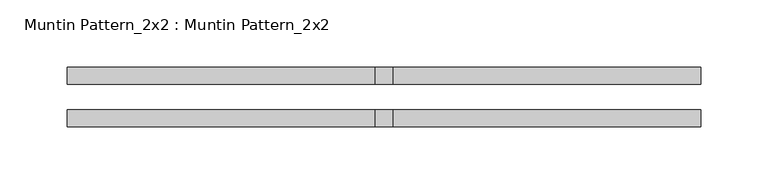
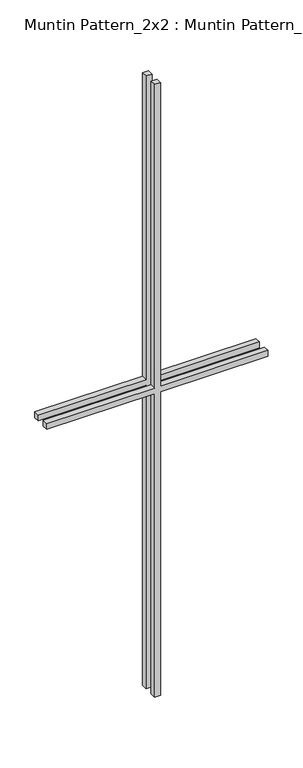
"""IFC4 building model written with IfcOpenShell, lengths in millimetres: proxy geometry, Muntin Pattern_2x2 : Muntin Pattern_2x2."""

from ifc_helpers import new_model, si_unit, frame, origin, place, context, project, spatial, polyline, outline, extrude, source, transform, mapped, element, save


def muntin_pattern_2x2_muntin_pattern_2x2_a30a3345(model_context):
    return source(origin(), model_context, "Body", "SweptSolid", [
        extrude(outline(polyline([(698.5, -6.35), (698.5, -236.5375), (685.8, -236.5375), (685.8, -6.35), (0.0, -6.35), (0.0, 6.35), (685.8, 6.35), (685.8, 236.5375), (698.5, 236.5375), (698.5, 6.35), (1384.3, 6.35), (1384.3, -6.35), (698.5, -6.35)])), frame((0.0, -22.225, 0.0), z_axis=(0.0, 1.0, 0.0), x_axis=(0.0, 0.0, 1.0)), (0.0, 0.0, 1.0), 12.7),
        extrude(outline(polyline([(698.5, -6.35), (698.5, -236.5375), (685.8, -236.5375), (685.8, -6.35), (0.0, -6.35), (0.0, 6.35), (685.8, 6.35), (685.8, 236.5375), (698.5, 236.5375), (698.5, 6.35), (1384.3, 6.35), (1384.3, -6.35), (698.5, -6.35)])), frame((0.0, 9.525, 0.0), z_axis=(0.0, 1.0, 0.0), x_axis=(0.0, 0.0, 1.0)), (0.0, 0.0, 1.0), 12.7),
    ])


if __name__ == "__main__":
    model = new_model("IFC4")
    model_context = context("Model", 3, world=origin())
    ifc_project = project(units=[si_unit("LENGTHUNIT", "METRE", prefix="MILLI")], contexts=[model_context])
    site = spatial("IfcSite", under=ifc_project)
    building = spatial("IfcBuilding", under=site)
    placement = place(None, origin())
    muntin_pattern_2x2_muntin_pattern_2x2_shape = muntin_pattern_2x2_muntin_pattern_2x2_a30a3345(model_context)
    element("IfcBuildingElementProxy", 1, Name="Muntin Pattern_2x2 : Muntin Pattern_2x2", ObjectType="Muntin Pattern_2x2 : Muntin Pattern_2x2", at=placement, inside=building, context=model_context, shape_type="MappedRepresentation", body=[
        mapped(muntin_pattern_2x2_muntin_pattern_2x2_shape, transform((0.0, 0.0, 0.0), x_axis=(1.0, 0.0, 0.0), y_axis=(0.0, 1.0, 0.0), z_axis=(0.0, 0.0, 1.0))),
    ])
    save(model, "model.ifc")

# Revit data of these elements
# Type "Muntin Pattern_2x2 : Muntin Pattern_2x2"
#   Width [instance default] = 4' - 0"
#   Thickness = 0' - 0 1/2"
#   Height [instance default] = 4' - 0"
#   Distance = 0' - 0 3/4"
#   Interior Material [instance default] = none
#   Exterior Material [instance default] = none
#   Default Elevation = 0
# Element 1 (IfcBuildingElementProxy, "Muntin Pattern_2x2 : Muntin Pattern_2x2")
#   Width = 1' - 6 5/8"
#   Height = 4' - 6 1/2"
#   Interior Material = Wood - Stained
#   Exterior Material = Clad - White
#   Materials on its faces: "Clad - White", "Wood - Stained"
# Materials
#   "Clad - White": class "Wood", colour RGB 242 242 238, transparency 0, Cost = 0
#   "Wood - Stained": class "Wood", colour RGB 224 178 126, transparency 0, Cost = 0
